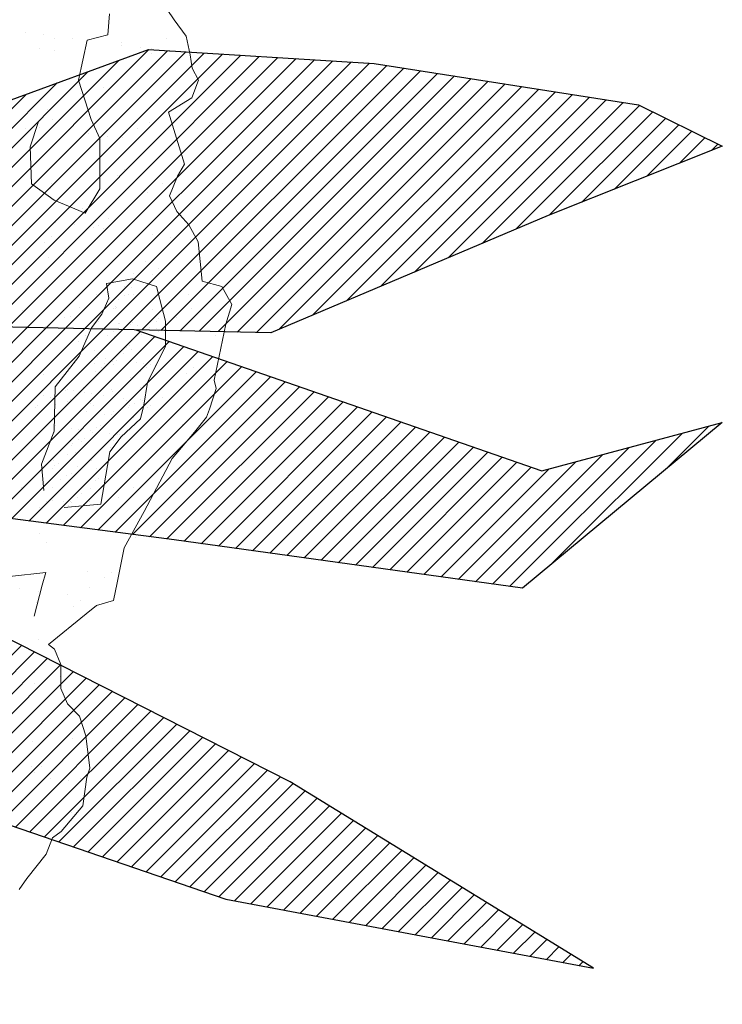
# Model space of a CAD drawing. Units: inches. Extents: x 1986 to 21484, y -1816 to 2016.
# Tile 31 of 85: x 2183.13 to 2190.96, y 1876.39 to 1887.36. Entities that reach past the tile are written whole.
import ezdxf

# ---------------------------------------------------------------- set-up
doc = ezdxf.new("R2010")
doc.units = ezdxf.units.IN
doc.layers.add('L-PLNT', color=84, linetype='Continuous', lineweight=13)
doc.layers.add('vfolhas', color=114, linetype='Continuous', lineweight=5)
for name, color, linetype in [('vfolha', 72, 'Continuous'), ('vfolha2', 110, 'Continuous'), ('vfolhas2', 102, 'Continuous')]:
    doc.layers.add(name, color=color, linetype=linetype)
pattern_1 = [(45, (-2446.5133113, 50.986076), (-0.004419417382, 0.004419417382), [])]

# ---------------------------------------------------------------- blocks, each defined once
blk = doc.blocks.new('arbusto_PB_verde_grande')
at = {"layer": 'vfolha2'}
h = blk.add_hatch(dxfattribs=at)
h.set_pattern_fill('ANSI31', color=256, scale=0.05, style=0)
h.set_pattern_definition(pattern_1)
h.paths.add_polyline_path([(0.02944, 0.35651), (0.00028, 0.09048), (0.02625, -0.03934), (0.047, 0.06233), (0.06189, 0.09731), (0.09372, 0.26573), (0.09955, 0.43473), (0.08789, 0.61313), (0.0645, 0.72266), (0.04988, 0.6851), (0.0236, 0.51294)])
h.paths.add_polyline_path([(0.30106, 0.43789), (0.14225, 0.24871), (0.26685, 0.30022)])
h.paths.add_polyline_path([(0.37995, 0.22817), (0.23697, 0.15193), (0.18428, 0.09364), (0.11122, 0.04358), (0.02625, -0.03934), (0.28061, 0.04667), (0.36829, 0.07798), (0.46756, 0.11239), (0.61068, 0.19376), (0.71585, 0.27823), (0.55813, 0.25948)])
h.paths.add_polyline_path([(0.56101, -0.29441), (0.72752, -0.32573), (0.59024, -0.2412), (0.42962, -0.15982), (0.02625, -0.03934), (0.14922, -0.14107), (0.18838, -0.16604), (0.41501, -0.24435)])
h.paths.add_polyline_path([(-0.27429, -0.44776), (-0.30352, -0.72628), (-0.23923, -0.64175), (-0.15457, -0.45716), (0.02625, -0.03934), (-0.16328, -0.25376)])
h.paths.add_polyline_path([(-0.51963, -0.24744), (-0.67736, -0.32573), (-0.59558, -0.35072), (-0.40574, -0.32882), (-0.21007, -0.20995), (0.02625, -0.03934), (-0.14874, -0.06595), (-0.31518, -0.09101), (-0.41452, -0.15048)])
h.paths.add_polyline_path([(-0.52546, 0.25007), (-0.70947, 0.24698), (-0.51963, 0.1093), (-0.32979, 0.02167), (-0.07567, -0.0128), (-0.04234, -0.02148), (-0.35024, 0.1312)])
at = {"layer": 'vfolhas'}
h = blk.add_hatch(dxfattribs=at)
h.set_pattern_fill('ANSI31', color=256, scale=0.05, style=0)
h.set_pattern_definition(pattern_1)
h.paths.add_polyline_path([(-0.07279, 0.50669), (-0.18085, 0.65063), (-0.2334, 0.67253), (-0.20712, 0.53176), (-0.10785, 0.25007), (0.02625, -0.03934), (0.00028, 0.09048), (0.00816, 0.16241), (-0.04939, 0.29079)])
h.paths.add_polyline_path([(0.09902, 0.41929), (0.09372, 0.26573), (0.07906, 0.18814), (0.15506, 0.36901), (0.26606, 0.5505), (0.28356, 0.63504), (0.2485, 0.68819), (0.25145, 0.63504), (0.20178, 0.54426)])
h.paths.add_polyline_path([(0.12295, 0.24073), (0.047, 0.06233), (0.02625, -0.03934), (0.11122, 0.04358), (0.18428, 0.09364), (0.27478, 0.19376), (0.3215, 0.25323), (0.44129, 0.38467), (0.47634, 0.57866), (0.41789, 0.45347), (0.28939, 0.30954)])
h.paths.add_polyline_path([(0.58145, -0.03779), (0.70707, 0.01536), (0.78591, 0.04667), (0.74796, 0.06549), (0.62818, 0.08423), (0.52595, 0.09048), (0.39745, 0.04358), (0.02625, -0.03934), (0.25728, -0.03154), (0.43834, -0.0347)])
h.paths.add_polyline_path([(0.52022, -0.03647), (0.43834, -0.0347), (0.25728, -0.03154), (0.02625, -0.03934), (0.17964, -0.08515), (0.53768, -0.13167), (0.69541, -0.15357), (0.78591, -0.07852), (0.70413, -0.10042)])
h.paths.add_polyline_path([(0.27189, -0.21929), (0.14922, -0.14107), (0.02625, -0.03934), (0.15794, -0.31007), (0.29522, -0.42585), (0.41789, -0.49157), (0.56396, -0.56669), (0.5114, -0.48532), (0.39456, -0.34139)])
h.paths.add_polyline_path([(-0.05818, -0.47591), (-0.02312, -0.61984), (0.047, -0.80134), (0.08494, -0.59794), (0.07911, -0.4071), (0.03527, -0.25376), (0.02625, -0.03934), (-0.03773, -0.26001)])
h.paths.add_polyline_path([(-0.24218, 0.14054), (-0.11073, 0.06858), (0.02625, -0.03934), (-0.04235, 0.10871), (-0.21007, 0.23757), (-0.36485, 0.33145), (-0.47874, 0.40341), (-0.54303, 0.46288), (-0.49041, 0.33145), (-0.39408, 0.22192)])
at = {"layer": 'vfolha'}
for p, q in [((0.52022, -0.03647), (0.70413, -0.10042)), ((0.78591, -0.07852), (0.69541, -0.15357)), ((0.70413, -0.10042), (0.78591, -0.07852)), ((0.53768, -0.13167), (0.17964, -0.08515)), ((0.69541, -0.15357), (0.53768, -0.13167))]:
    blk.add_line(p, q, dxfattribs=at)
at = {"layer": 'vfolha2'}
for p, q in [((0.59024, -0.2412), (0.42962, -0.15982)), ((0.41501, -0.24435), (0.56101, -0.29441)), ((0.72752, -0.32573), (0.59024, -0.2412)), ((0.56101, -0.29441), (0.72752, -0.32573))]:
    blk.add_line(p, q, dxfattribs=at)
at = {"layer": 'vfolhas2'}
for p, q in [((0.39745, 0.04358), (0.52595, 0.09048)), ((0.52595, 0.09048), (0.62818, 0.08423)), ((0.62818, 0.08423), (0.74796, 0.06549)), ((0.74796, 0.06549), (0.78591, 0.04667)), ((0.78591, 0.04667), (0.70707, 0.01536)), ((0.70707, 0.01536), (0.58145, -0.03779)), ((0.58145, -0.03779), (0.43834, -0.0347))]:
    blk.add_line(p, q, dxfattribs=at)
blk = doc.blocks.new('PLANT-SHRUB')
for p, q in [((2184.684, 1887.612), (2184.851, 1887.364)), ((2184.129, 1887.429), (2184.111, 1887.195)), ((2184.851, 1887.364), (2184.984, 1887.18)), ((2183.19, 1887.223), (2183.19, 1887.223)), ((2183.398, 1887.196), (2183.398, 1887.196)), ((2183.518, 1887.156), (2183.518, 1887.156)), ((2183.723, 1887.153), (2183.723, 1887.153)), ((2184.111, 1887.195), (2183.88, 1887.136)), ((2184.763, 1887.154), (2184.763, 1887.154)), ((2184.984, 1887.18), (2185.03, 1886.972)), ((2183.35, 1887.049), (2183.35, 1887.049)), ((2183.88, 1887.136), (2183.785, 1886.689)), ((2184.264, 1887.115), (2184.264, 1887.115)), ((2184.266, 1887.082), (2184.266, 1887.082)), ((2184.474, 1887.054), (2184.474, 1887.054)), ((2184.594, 1887.047), (2184.594, 1887.047)), ((2183.522, 1887.023), (2183.522, 1887.023)), ((2184.601, 1886.984), (2184.601, 1886.984)), ((2184.799, 1887.012), (2184.799, 1887.012)), ((2185.03, 1886.972), (2185.053, 1886.823)), ((2185.053, 1886.823), (2185.122, 1886.69)), ((2183.842, 1886.729), (2183.842, 1886.729)), ((2183.916, 1886.797), (2183.916, 1886.797)), ((2183.785, 1886.689), (2183.926, 1886.251)), ((2183.785, 1886.689), (2183.785, 1886.689)), ((2184.061, 1886.61), (2184.061, 1886.61)), ((2185.122, 1886.69), (2185.047, 1886.494)), ((2183.802, 1886.542), (2183.802, 1886.542)), ((2185.047, 1886.494), (2184.788, 1886.333)), ((2183.444, 1886.365), (2183.444, 1886.365)), ((2184.788, 1886.333), (2184.967, 1885.753)), ((2184.788, 1886.333), (2184.788, 1886.333)), ((2183.244, 1885.949), (2183.334, 1886.22)), ((2183.355, 1886.167), (2183.355, 1886.167)), ((2183.497, 1886.253), (2183.497, 1886.253)), ((2183.926, 1886.251), (2184.021, 1886.039)), ((2184.576, 1886.214), (2184.576, 1886.214)), ((2183.196, 1886.156), (2183.196, 1886.156)), ((2183.897, 1886.095), (2183.897, 1886.095)), ((2184.105, 1886.068), (2184.105, 1886.068)), ((2184.44, 1886.153), (2184.44, 1886.153)), ((2183.262, 1885.534), (2183.244, 1885.949)), ((2184.021, 1886.039), (2184.021, 1885.714)), ((2184.272, 1886.046), (2184.272, 1886.046)), ((2184.43, 1886.025), (2184.43, 1886.025)), ((2184.646, 1886.014), (2184.646, 1886.014)), ((2184.036, 1885.84), (2184.036, 1885.84)), ((2184.967, 1885.753), (2184.886, 1885.62)), ((2184.021, 1885.714), (2184.021, 1885.479)), ((2184.224, 1885.628), (2184.224, 1885.628)), ((2184.298, 1885.695), (2184.298, 1885.695)), ((2184.886, 1885.62), (2184.799, 1885.401)), ((2183.515, 1885.353), (2183.262, 1885.534)), ((2183.48, 1885.541), (2183.48, 1885.541)), ((2184.724, 1885.539), (2184.724, 1885.539)), ((2183.472, 1885.483), (2183.472, 1885.483)), ((2184.021, 1885.479), (2183.858, 1885.209)), ((2184.551, 1885.444), (2184.551, 1885.444)), ((2184.799, 1885.401), (2184.88, 1885.228)), ((2183.858, 1885.209), (2183.515, 1885.353)), ((2183.827, 1885.263), (2183.827, 1885.263)), ((2183.858, 1885.209), (2183.858, 1885.209)), ((2184.88, 1885.228), (2185.013, 1885.078)), ((2183.529, 1885.109), (2183.529, 1885.109)), ((2183.737, 1885.082), (2183.737, 1885.082)), ((2184.011, 1885.069), (2184.011, 1885.069)), ((2184.117, 1885.152), (2184.117, 1885.152)), ((2185.013, 1885.078), (2185.117, 1884.888)), ((2183.949, 1885.045), (2183.949, 1885.045)), ((2184.062, 1885.039), (2184.062, 1885.039)), ((2184.605, 1884.968), (2184.605, 1884.968)), ((2183.405, 1884.877), (2183.405, 1884.877)), ((2183.479, 1884.945), (2183.479, 1884.945)), ((2184.813, 1884.94), (2184.813, 1884.94)), ((2185.028, 1884.913), (2185.028, 1884.913)), ((2185.117, 1884.888), (2185.163, 1884.45)), ((2183.446, 1884.713), (2183.446, 1884.713)), ((2184.526, 1884.674), (2184.526, 1884.674)), ((2183.157, 1884.54), (2183.157, 1884.54)), ((2184.401, 1884.538), (2184.401, 1884.538)), ((2184.607, 1884.526), (2184.607, 1884.526)), ((2184.68, 1884.594), (2184.68, 1884.594)), ((2184.387, 1884.475), (2184.095, 1884.424)), ((2184.095, 1884.424), (2184.121, 1884.259)), ((2184.387, 1884.475), (2184.387, 1884.475)), ((2184.654, 1884.389), (2184.387, 1884.475)), ((2185.163, 1884.45), (2185.382, 1884.392)), ((2185.163, 1884.45), (2185.163, 1884.45)), ((2183.986, 1884.299), (2183.986, 1884.299)), ((2184.293, 1884.388), (2184.293, 1884.388)), ((2184.338, 1884.301), (2184.338, 1884.301)), ((2184.377, 1884.377), (2184.377, 1884.377)), ((2184.396, 1884.3), (2184.396, 1884.3)), ((2184.507, 1884.36), (2184.507, 1884.36)), ((2184.691, 1884.247), (2184.654, 1884.389)), ((2185.008, 1884.304), (2185.008, 1884.304)), ((2185.382, 1884.392), (2185.492, 1884.19)), ((2184.121, 1884.259), (2184.045, 1884.082)), ((2184.235, 1884.244), (2184.235, 1884.244)), ((2184.302, 1884.287), (2184.302, 1884.287)), ((2184.755, 1884.006), (2184.691, 1884.247)), ((2185.492, 1884.19), (2185.428, 1883.971)), ((2183.16, 1884.123), (2183.16, 1884.123)), ((2183.368, 1884.095), (2183.368, 1884.095)), ((2183.795, 1884.152), (2183.795, 1884.152)), ((2184.045, 1884.082), (2183.931, 1883.93)), ((2184.17, 1884.146), (2184.17, 1884.146)), ((2184.194, 1884.14), (2184.194, 1884.14)), ((2184.199, 1884.173), (2184.199, 1884.173)), ((2184.209, 1884.162), (2184.209, 1884.162)), ((2184.612, 1884.134), (2184.612, 1884.134)), ((2185.039, 1884.149), (2185.039, 1884.149)), ((2183.626, 1884.044), (2183.626, 1884.044)), ((2183.693, 1884.053), (2183.693, 1884.053)), ((2183.977, 1883.99), (2183.977, 1883.99)), ((2184.011, 1884), (2184.011, 1884)), ((2184.146, 1883.993), (2184.146, 1883.993)), ((2184.229, 1883.982), (2184.229, 1883.982)), ((2184.236, 1883.981), (2184.236, 1883.981)), ((2184.386, 1883.992), (2184.386, 1883.992)), ((2184.416, 1884.041), (2184.416, 1884.041)), ((2184.651, 1884.006), (2184.651, 1884.006)), ((2184.68, 1884.033), (2184.68, 1884.033)), ((2184.755, 1884.006), (2184.755, 1884.006)), ((2184.755, 1883.727), (2184.755, 1884.006)), ((2184.871, 1884.042), (2184.871, 1884.042)), ((2185.428, 1883.971), (2185.296, 1883.345)), ((2183.421, 1883.943), (2183.421, 1883.943)), ((2183.931, 1883.93), (2183.791, 1883.613)), ((2184.173, 1883.887), (2184.173, 1883.887)), ((2184.359, 1883.965), (2184.359, 1883.965)), ((2184.444, 1883.954), (2184.444, 1883.954)), ((2184.491, 1883.86), (2184.491, 1883.86)), ((2184.501, 1883.904), (2184.501, 1883.904)), ((2184.576, 1883.936), (2184.576, 1883.936)), ((2184.659, 1883.926), (2184.659, 1883.926)), ((2184.671, 1883.886), (2184.671, 1883.886)), ((2184.769, 1883.911), (2184.769, 1883.911)), ((2183.788, 1883.776), (2183.788, 1883.776)), ((2183.861, 1883.843), (2183.861, 1883.843)), ((2184.105, 1883.844), (2184.105, 1883.844)), ((2184.183, 1883.832), (2184.183, 1883.832)), ((2184.602, 1883.826), (2184.602, 1883.826)), ((2184.603, 1883.843), (2184.603, 1883.843)), ((2185.312, 1883.84), (2185.312, 1883.84)), ((2183.967, 1883.682), (2183.967, 1883.682)), ((2184.286, 1883.641), (2184.286, 1883.641)), ((2184.323, 1883.706), (2184.323, 1883.706)), ((2184.352, 1883.733), (2184.352, 1883.733)), ((2184.376, 1883.684), (2184.376, 1883.684)), ((2184.552, 1883.322), (2184.755, 1883.727)), ((2183.791, 1883.613), (2183.525, 1883.271)), ((2183.742, 1883.539), (2183.742, 1883.539)), ((2183.96, 1883.529), (2183.96, 1883.529)), ((2183.999, 1883.599), (2183.999, 1883.599)), ((2184.079, 1883.537), (2184.079, 1883.537)), ((2184.082, 1883.588), (2184.082, 1883.588)), ((2184.164, 1883.56), (2184.164, 1883.56)), ((2184.212, 1883.571), (2184.212, 1883.571)), ((2184.429, 1883.542), (2184.429, 1883.542)), ((2184.512, 1883.531), (2184.512, 1883.531)), ((2184.983, 1883.534), (2184.983, 1883.534)), ((2183.976, 1883.443), (2183.976, 1883.443)), ((2184.025, 1883.432), (2184.025, 1883.432)), ((2184.044, 1883.486), (2184.044, 1883.486)), ((2184.173, 1883.524), (2184.173, 1883.524)), ((2184.474, 1883.442), (2184.474, 1883.442)), ((2184.542, 1883.485), (2184.542, 1883.485)), ((2184.592, 1883.518), (2184.592, 1883.518)), ((2184.642, 1883.514), (2184.642, 1883.514)), ((2184.989, 1883.425), (2184.989, 1883.425)), ((2185.063, 1883.493), (2185.063, 1883.493)), ((2183.39, 1883.411), (2183.39, 1883.411)), ((2183.957, 1883.374), (2183.957, 1883.374)), ((2183.995, 1883.405), (2183.995, 1883.405)), ((2184.366, 1883.376), (2184.366, 1883.376)), ((2184.514, 1883.068), (2184.552, 1883.322)), ((2185.296, 1883.345), (2185.319, 1883.253)), ((2183.525, 1883.271), (2183.512, 1882.777)), ((2183.525, 1883.271), (2183.525, 1883.271)), ((2183.634, 1883.233), (2183.634, 1883.233)), ((2183.659, 1883.241), (2183.659, 1883.241)), ((2183.732, 1883.231), (2183.732, 1883.231)), ((2183.836, 1883.26), (2183.836, 1883.26)), ((2183.851, 1883.204), (2183.851, 1883.204)), ((2184.157, 1883.241), (2184.157, 1883.241)), ((2184.163, 1883.216), (2184.163, 1883.216)), ((2184.476, 1883.265), (2184.476, 1883.265)), ((2184.505, 1883.292), (2184.505, 1883.292)), ((2185.319, 1883.253), (2185.244, 1883.022)), ((2183.396, 1883.173), (2183.396, 1883.173)), ((2183.472, 1883.151), (2183.472, 1883.151)), ((2183.667, 1883.105), (2183.667, 1883.105)), ((2183.697, 1883.132), (2183.697, 1883.132)), ((2183.934, 1883.193), (2183.934, 1883.193)), ((2184.064, 1883.176), (2184.064, 1883.176)), ((2184.281, 1883.147), (2184.281, 1883.147)), ((2184.317, 1883.119), (2184.317, 1883.119)), ((2184.365, 1883.136), (2184.365, 1883.136)), ((2184.476, 1883.134), (2184.476, 1883.134)), ((2184.495, 1883.119), (2184.495, 1883.119)), ((2184.717, 1883.149), (2184.717, 1883.149)), ((2183.303, 1883.043), (2183.303, 1883.043)), ((2183.325, 1883.066), (2183.325, 1883.066)), ((2183.529, 1883.071), (2183.529, 1883.071)), ((2183.847, 1883.043), (2183.847, 1883.043)), ((2183.868, 1882.995), (2183.868, 1882.995)), ((2183.915, 1883.086), (2183.915, 1883.086)), ((2183.947, 1883.066), (2183.947, 1883.066)), ((2184.178, 1882.992), (2184.178, 1882.992)), ((2184.345, 1883.042), (2184.345, 1883.042)), ((2184.356, 1883.068), (2184.356, 1883.068)), ((2184.412, 1883.085), (2184.412, 1883.085)), ((2184.476, 1882.916), (2184.514, 1883.068)), ((2184.514, 1883.068), (2184.514, 1883.068)), ((2184.548, 1883.041), (2184.548, 1883.041)), ((2184.591, 1883.061), (2184.591, 1883.061)), ((2185.244, 1883.022), (2185.21, 1882.935)), ((2183.721, 1882.923), (2183.721, 1882.923)), ((2184.076, 1882.968), (2184.076, 1882.968)), ((2184.148, 1882.965), (2184.148, 1882.965)), ((2184.153, 1882.908), (2184.153, 1882.908)), ((2184.26, 1882.713), (2184.476, 1882.916)), ((2184.401, 1882.925), (2184.401, 1882.925)), ((2185.21, 1882.935), (2185.077, 1882.768)), ((2183.512, 1882.777), (2183.373, 1882.409)), ((2183.512, 1882.777), (2183.512, 1882.777)), ((2183.519, 1882.763), (2183.519, 1882.763)), ((2183.53, 1882.841), (2183.53, 1882.841)), ((2183.704, 1882.81), (2183.704, 1882.81)), ((2183.787, 1882.799), (2183.787, 1882.799)), ((2183.917, 1882.782), (2183.917, 1882.782)), ((2183.935, 1882.759), (2183.935, 1882.759)), ((2183.989, 1882.819), (2183.989, 1882.819)), ((2184.028, 1882.84), (2184.028, 1882.84)), ((2185.077, 1882.768), (2184.829, 1882.474)), ((2184.944, 1882.853), (2184.944, 1882.853)), ((2183.786, 1882.686), (2183.786, 1882.686)), ((2183.82, 1882.665), (2183.82, 1882.665)), ((2183.85, 1882.692), (2183.85, 1882.692)), ((2183.937, 1882.758), (2183.937, 1882.758)), ((2184.133, 1882.549), (2184.26, 1882.713)), ((2184.134, 1882.753), (2184.134, 1882.753)), ((2184.17, 1882.674), (2184.17, 1882.674)), ((2184.217, 1882.742), (2184.217, 1882.742)), ((2184.244, 1882.742), (2184.244, 1882.742)), ((2183.711, 1882.615), (2183.711, 1882.615)), ((2183.718, 1882.643), (2183.718, 1882.643)), ((2184.108, 1882.397), (2184.133, 1882.549)), ((2184.143, 1882.6), (2184.143, 1882.6)), ((2183.401, 1882.441), (2183.401, 1882.441)), ((2183.509, 1882.455), (2183.509, 1882.455)), ((2183.661, 1882.519), (2183.661, 1882.519)), ((2183.756, 1882.537), (2183.756, 1882.537)), ((2183.899, 1882.44), (2183.899, 1882.44)), ((2183.927, 1882.45), (2183.927, 1882.45)), ((2184.829, 1882.474), (2184.517, 1881.881)), ((2183.371, 1882.403), (2183.371, 1882.403)), ((2183.373, 1882.409), (2183.398, 1882.118)), ((2183.373, 1882.409), (2183.373, 1882.409)), ((2183.493, 1882.364), (2183.493, 1882.364)), ((2183.522, 1882.391), (2183.522, 1882.391)), ((2183.556, 1882.415), (2183.556, 1882.415)), ((2183.64, 1882.404), (2183.64, 1882.404)), ((2183.77, 1882.387), (2183.77, 1882.387)), ((2183.987, 1882.358), (2183.987, 1882.358)), ((2184.032, 1881.966), (2184.108, 1882.397)), ((2184.07, 1882.347), (2184.07, 1882.347)), ((2184.45, 1882.364), (2184.45, 1882.364)), ((2183.589, 1882.242), (2183.589, 1882.242)), ((2183.656, 1882.285), (2183.656, 1882.285)), ((2183.701, 1882.307), (2183.701, 1882.307)), ((2183.772, 1882.31), (2183.772, 1882.31)), ((2183.973, 1882.224), (2183.973, 1882.224)), ((2184.003, 1882.251), (2184.003, 1882.251)), ((2183.149, 1882.15), (2183.149, 1882.15)), ((2183.398, 1882.118), (2183.398, 1882.118)), ((2183.498, 1882.147), (2183.498, 1882.147)), ((2183.917, 1882.142), (2183.917, 1882.142)), ((2184.394, 1882.148), (2184.394, 1882.148)), ((2183.424, 1881.991), (2183.424, 1881.991)), ((2183.499, 1882.009), (2183.499, 1882.009)), ((2183.622, 1881.992), (2183.622, 1881.992)), ((2183.691, 1881.999), (2183.691, 1881.999)), ((2183.77, 1882.04), (2183.77, 1882.04)), ((2183.814, 1882.078), (2183.814, 1882.078)), ((2184.225, 1882.04), (2184.225, 1882.04)), ((2183.351, 1881.924), (2183.351, 1881.924)), ((2183.626, 1881.928), (2184.032, 1881.966)), ((2183.675, 1881.951), (2183.675, 1881.951)), ((2183.707, 1881.981), (2183.707, 1881.981)), ((2183.839, 1881.964), (2183.839, 1881.964)), ((2183.91, 1881.989), (2183.91, 1881.989)), ((2184.032, 1881.938), (2184.032, 1881.938)), ((2184.517, 1881.881), (2184.292, 1881.477)), ((2183.346, 1881.633), (2183.346, 1881.633)), ((2184.425, 1881.594), (2184.425, 1881.594)), ((2183.433, 1881.536), (2183.433, 1881.536)), ((2184.292, 1881.477), (2184.216, 1881.087)), ((2183.014, 1881.159), (2183.422, 1881.204)), ((2183.422, 1881.204), (2183.378, 1881.062)), ((2183.885, 1881.219), (2183.885, 1881.219)), ((2184.071, 1881.147), (2184.071, 1881.147)), ((2184.154, 1881.208), (2184.154, 1881.208)), ((2183.131, 1881.022), (2183.131, 1881.022)), ((2183.378, 1881.062), (2183.289, 1880.716)), ((2183.902, 1881.04), (2183.902, 1881.04)), ((2184.216, 1881.087), (2184.176, 1880.891)), ((2183.339, 1880.995), (2183.339, 1880.995)), ((2183.664, 1880.952), (2183.664, 1880.952)), ((2183.321, 1880.863), (2183.321, 1880.863)), ((2183.733, 1880.822), (2183.733, 1880.822)), ((2183.807, 1880.89), (2183.807, 1880.89)), ((2183.986, 1880.834), (2183.87, 1880.741)), ((2184.176, 1880.891), (2183.986, 1880.834)), ((2183.87, 1880.741), (2183.449, 1880.401)), ((2183.335, 1880.458), (2183.335, 1880.458)), ((2183.449, 1880.401), (2183.518, 1880.349)), ((2183.518, 1880.349), (2183.588, 1880.176)), ((2183.588, 1880.176), (2183.588, 1879.911)), ((2183.295, 1880.092), (2183.295, 1880.092)), ((2183.58, 1880.039), (2183.58, 1880.039)), ((2183.295, 1879.966), (2183.295, 1879.966)), ((2183.588, 1879.911), (2183.663, 1879.738)), ((2183.663, 1879.738), (2183.795, 1879.6)), ((2183.795, 1879.6), (2183.865, 1879.381)), ((2183.717, 1879.356), (2183.717, 1879.356)), ((2183.865, 1879.381), (2183.909, 1879.023)), ((2183.27, 1879.322), (2183.27, 1879.322)), ((2183.425, 1879.145), (2183.425, 1879.145)), ((2183.257, 1879.038), (2183.257, 1879.038)), ((2183.37, 1879.038), (2183.37, 1879.038)), ((2183.296, 1878.97), (2183.296, 1878.97)), ((2183.877, 1878.92), (2183.831, 1878.602)), ((2183.909, 1879.023), (2183.877, 1878.92)), ((2183.47, 1878.908), (2183.47, 1878.908)), ((2183.678, 1878.881), (2183.678, 1878.881)), ((2183.809, 1878.909), (2183.809, 1878.909)), ((2183.831, 1878.602), (2183.591, 1878.317)), ((2183.245, 1878.552), (2183.245, 1878.552)), ((2183.709, 1878.531), (2183.709, 1878.531)), ((2183.591, 1878.317), (2183.494, 1878.246)), ((2183.494, 1878.246), (2183.423, 1878.064)), ((2183.423, 1878.064), (2183.209, 1877.792)), ((2183.209, 1877.792), (2183.124, 1877.669))]:
    blk.add_line(p, q)

msp = doc.modelspace()

# ---------------------------------------------------------------- block references
at = {"layer": 'L-PLNT'}
msp.add_blockref('PLANT-SHRUB', (0, 0), dxfattribs=at)
at = {"layer": 'L-PLNT', "xscale": 24.60366729364114, "yscale": 24.60366729364114, "zscale": 24.60366729364114}
msp.add_blockref('arbusto_PB_verde_grande', (2171.623, 1884.805), dxfattribs=at)

doc.saveas('drawing.dxf')
